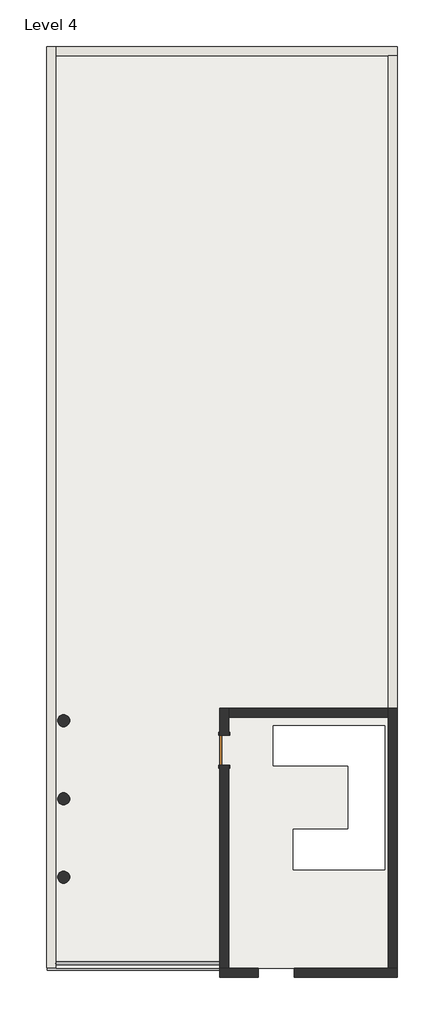
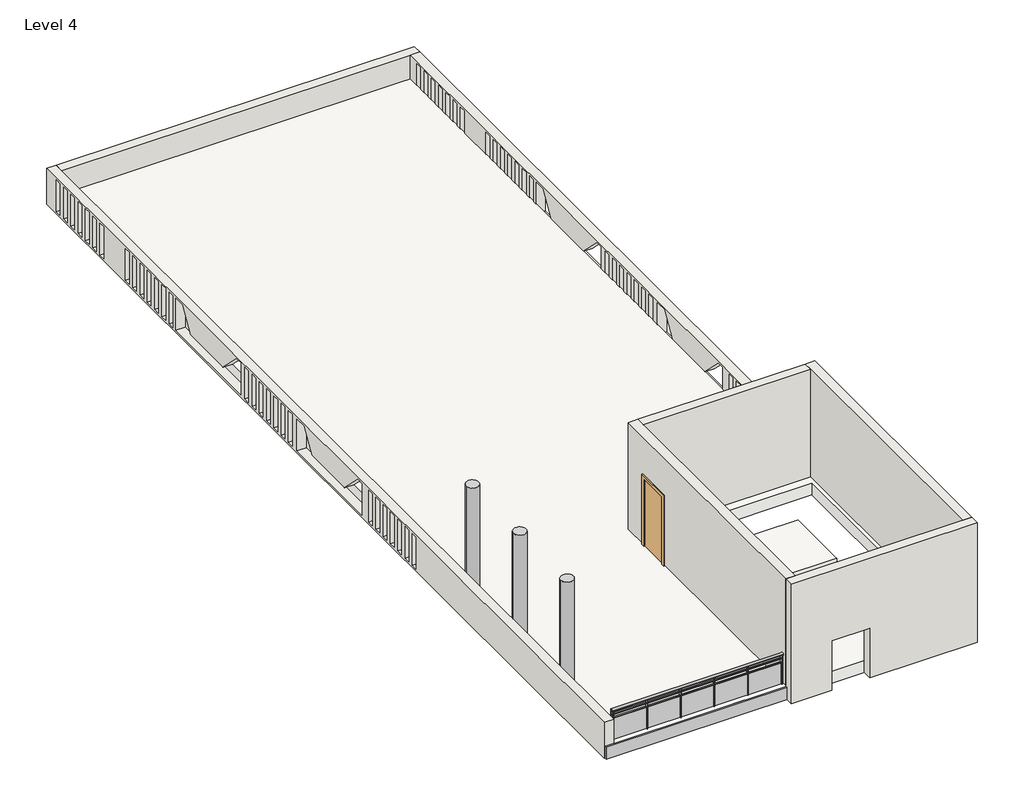
# One storey: 7 walls, 3 columns, 1 door, 1 proxy, 1 railing, 1 roof.
"""IFC4 building model written with IfcOpenShell, lengths in millimetres."""

from ifc_helpers import new_model, si_unit, point, frame, origin, place, context, project, spatial, polyline, ellipse_curve, trimmed, outline, extrude, faceted_brep, transform, mapped, element, save
from ifc_brep_helpers import plane_surface, extruded_surface, advanced_brep
from components import generic_models_12_generic_models_12_e4f72901, round_column_column_1_x_1_faae7945, door_a1484949

model = new_model("IFC4")

# Units and contexts
model_context = context("Model", 3, world=origin())
ifc_project = project(units=[si_unit("LENGTHUNIT", "METRE", prefix="MILLI")], contexts=[model_context])

# Site, building, storey
site = spatial("IfcSite", under=ifc_project)
building = spatial("IfcBuilding", under=site)
storey = spatial("IfcBuildingStorey", under=building, Name="Level 4", Elevation=6400.8)

# Proxy
placement = place(None, origin())
generic_models_12_generic_models_12_shape = generic_models_12_generic_models_12_e4f72901(model_context)
element("IfcBuildingElementProxy", 1, Name="Generic Models 12 : Generic Models 12", ObjectType="Generic Models 12 : Generic Models 12", at=placement, inside=storey, context=model_context, shape_type="MappedRepresentation", body=[
    mapped(generic_models_12_generic_models_12_shape, transform((0.0, 0.0, 0.0), x_axis=(1.0, 0.0, 0.0), y_axis=(0.0, 1.0, 0.0), z_axis=(0.0, 0.0, 1.0))),
])

# Columns
round_column_column_1_x_1_shape = round_column_column_1_x_1_faae7945(model_context)
element("IfcColumn", 2, ObjectType="Round Column : COLUMN 1' X 1'", at=placement, inside=storey, context=model_context, shape_type="MappedRepresentation", body=[
    mapped(round_column_column_1_x_1_shape, transform((1692.4423568, -10961.9073314, 0.0), x_axis=(1.0, 0.0, 0.0), y_axis=(0.0, 1.0, 0.0), z_axis=(0.0, 0.0, 1.0))),
])
element("IfcColumn", 3, ObjectType="Round Column : COLUMN 1' X 1'", at=placement, inside=storey, context=model_context, shape_type="MappedRepresentation", body=[
    mapped(round_column_column_1_x_1_shape, transform((1692.4423568, -6999.5073314, 0.0), x_axis=(1.0, 0.0, 0.0), y_axis=(0.0, 1.0, 0.0), z_axis=(0.0, 0.0, 1.0))),
])
element("IfcColumn", 4, ObjectType="Round Column : COLUMN 1' X 1'", at=placement, inside=storey, context=model_context, shape_type="MappedRepresentation", body=[
    mapped(round_column_column_1_x_1_shape, transform((1692.4423568, -8980.7073314, 0.0), x_axis=(1.0, 0.0, 0.0), y_axis=(0.0, 1.0, 0.0), z_axis=(0.0, 0.0, 1.0))),
])

# Door
door_shape = door_a1484949(model_context)
element("IfcDoor", 5, ObjectType="Single-Flush : 30\" x 80\"", at=placement, inside=storey, context=model_context, shape_type="MappedRepresentation", body=[
    mapped(door_shape, transform((5756.4423568, -7748.8073314, 6400.8), x_axis=(0.0, 1.0, 0.0), y_axis=(-1.0, 0.0, 0.0), z_axis=(0.0, 0.0, 1.0))),
])

# Railing
element("IfcRailing", 6, ObjectType="Glass Panel - Bottom Fill", at=placement, inside=storey, context=model_context, shape_type="SolidModel", body=[
    advanced_brep(
    [(1501.9423568, -13108.2073314, 7467.6), (1501.9423568, -13184.4073314, 7467.6), (5642.1423568, -13108.2073314, 7467.6), (5642.1423568, -13184.4073314, 7467.6)],
    [
        (0, 1, ellipse_curve(frame((1501.9423568, -13146.3073314, 7467.6), z_axis=(-1.0, 0.0, 0.0), x_axis=(0.0, -1.0, 0.0)), 38.1, 28.575)),
        (1, 0, ellipse_curve(frame((1501.9423568, -13146.3073314, 7467.6), z_axis=(-1.0, 0.0, 0.0), x_axis=(0.0, -1.0, 0.0)), 38.1, 28.575)),
        (2, 3, ellipse_curve(frame((5642.1423568, -13146.3073314, 7467.6), z_axis=(1.0, 0.0, 0.0), x_axis=(0.0, -1.0, 0.0)), 38.1, 28.575)),
        (3, 2, ellipse_curve(frame((5642.1423568, -13146.3073314, 7467.6), z_axis=(1.0, 0.0, 0.0), x_axis=(0.0, -1.0, 0.0)), 38.1, 28.575)),
        (0, 2),
        (3, 1),
    ],
    [
        plane_surface(frame((1501.9423568, -13146.3073314, 7467.6), z_axis=(-1.0, 0.0, 0.0), x_axis=(0.0, 1.0, 0.0))),
        plane_surface(frame((5642.1423568, -13146.3073314, 7467.6), z_axis=(1.0, 0.0, 0.0), x_axis=(0.0, 1.0, 0.0))),
        extruded_surface(trimmed(ellipse_curve(frame((5642.1423568, -13146.3073314, 7467.6), z_axis=(-1.0, 0.0, 0.0), x_axis=(0.0, -1.0, 0.0)), 38.1, 28.575), [point((5642.1423568, -13108.2073314, 7467.6))], [point((5642.1423568, -13184.4073314, 7467.6))], True, "CARTESIAN"), (-4140.2, 0.0, 0.0), 4140.2),
        extruded_surface(trimmed(ellipse_curve(frame((5642.1423568, -13146.3073314, 7467.6), z_axis=(-1.0, 0.0, 0.0), x_axis=(0.0, -1.0, 0.0)), 38.1, 28.575), [point((5642.1423568, -13184.4073314, 7467.6))], [point((5642.1423568, -13108.2073314, 7467.6))], True, "CARTESIAN"), (-4140.2, 0.0, 0.0), 4140.2),
    ],
    [
        (0, [[1, 2]]),
        (1, [[3, 4]]),
        (2, [[-1, 5, -4, 6]]),
        (3, [[-2, -6, -3, -5]]),
    ],
),
    extrude(outline(polyline([(1501.9423568, -13159.0073314), (1501.9423568, -13133.6073314), (5642.1423568, -13133.6073314), (5642.1423568, -13159.0073314), (1501.9423568, -13159.0073314)])), frame((0.0, 0.0, 7353.3), z_axis=(0.0, 0.0, 1.0), x_axis=(1.0, 0.0, 0.0)), (0.0, 0.0, 1.0), 25.4),
    extrude(outline(polyline([(1501.9423568, -13159.0073314), (1501.9423568, -13133.6073314), (5642.1423568, -13133.6073314), (5642.1423568, -13159.0073314), (1501.9423568, -13159.0073314)])), frame((0.0, 0.0, 7251.7), z_axis=(0.0, 0.0, 1.0), x_axis=(1.0, 0.0, 0.0)), (0.0, 0.0, 1.0), 25.4),
    extrude(outline(polyline([(5597.6923568, -13171.7073314), (5597.6923568, -13120.9073314), (5610.3923568, -13120.9073314), (5610.3923568, -13171.7073314), (5597.6923568, -13171.7073314)])), frame((0.0, 0.0, 6553.2), z_axis=(0.0, 0.0, 1.0), x_axis=(1.0, 0.0, 0.0)), (0.0, 0.0, 1.0), 885.825),
    extrude(outline(polyline([(4791.2423568, -13139.7721744), (5604.0423568, -13139.7721744), (5604.0423568, -13146.1221744), (4791.2423568, -13146.1221744), (4791.2423568, -13139.7721744)])), frame((0.0, 0.0, 6654.8), z_axis=(0.0, 0.0, 1.0), x_axis=(1.0, 0.0, 0.0)), (0.0, 0.0, 1.0), 596.9),
    extrude(outline(polyline([(4784.8923568, -13171.7073314), (4784.8923568, -13120.9073314), (4797.5923568, -13120.9073314), (4797.5923568, -13171.7073314), (4784.8923568, -13171.7073314)])), frame((0.0, 0.0, 6553.2), z_axis=(0.0, 0.0, 1.0), x_axis=(1.0, 0.0, 0.0)), (0.0, 0.0, 1.0), 885.825),
    extrude(outline(polyline([(3978.4423568, -13139.7721744), (4791.2423568, -13139.7721744), (4791.2423568, -13146.1221744), (3978.4423568, -13146.1221744), (3978.4423568, -13139.7721744)])), frame((0.0, 0.0, 6654.8), z_axis=(0.0, 0.0, 1.0), x_axis=(1.0, 0.0, 0.0)), (0.0, 0.0, 1.0), 596.9),
    extrude(outline(polyline([(3972.0923568, -13171.7073314), (3972.0923568, -13120.9073314), (3984.7923568, -13120.9073314), (3984.7923568, -13171.7073314), (3972.0923568, -13171.7073314)])), frame((0.0, 0.0, 6553.2), z_axis=(0.0, 0.0, 1.0), x_axis=(1.0, 0.0, 0.0)), (0.0, 0.0, 1.0), 885.825),
    extrude(outline(polyline([(3165.6423568, -13139.7721744), (3978.4423568, -13139.7721744), (3978.4423568, -13146.1221744), (3165.6423568, -13146.1221744), (3165.6423568, -13139.7721744)])), frame((0.0, 0.0, 6654.8), z_axis=(0.0, 0.0, 1.0), x_axis=(1.0, 0.0, 0.0)), (0.0, 0.0, 1.0), 596.9),
    extrude(outline(polyline([(3159.2923568, -13171.7073314), (3159.2923568, -13120.9073314), (3171.9923568, -13120.9073314), (3171.9923568, -13171.7073314), (3159.2923568, -13171.7073314)])), frame((0.0, 0.0, 6553.2), z_axis=(0.0, 0.0, 1.0), x_axis=(1.0, 0.0, 0.0)), (0.0, 0.0, 1.0), 885.825),
    extrude(outline(polyline([(2352.8423568, -13139.7721744), (3165.6423568, -13139.7721744), (3165.6423568, -13146.1221744), (2352.8423568, -13146.1221744), (2352.8423568, -13139.7721744)])), frame((0.0, 0.0, 6654.8), z_axis=(0.0, 0.0, 1.0), x_axis=(1.0, 0.0, 0.0)), (0.0, 0.0, 1.0), 596.9),
    extrude(outline(polyline([(2346.4923568, -13171.7073314), (2346.4923568, -13120.9073314), (2359.1923568, -13120.9073314), (2359.1923568, -13171.7073314), (2346.4923568, -13171.7073314)])), frame((0.0, 0.0, 6553.2), z_axis=(0.0, 0.0, 1.0), x_axis=(1.0, 0.0, 0.0)), (0.0, 0.0, 1.0), 885.825),
    extrude(outline(polyline([(1540.0423568, -13139.7721744), (2352.8423568, -13139.7721744), (2352.8423568, -13146.1221744), (1540.0423568, -13146.1221744), (1540.0423568, -13139.7721744)])), frame((0.0, 0.0, 6654.8), z_axis=(0.0, 0.0, 1.0), x_axis=(1.0, 0.0, 0.0)), (0.0, 0.0, 1.0), 596.9),
    extrude(outline(polyline([(1533.6923568, -13171.7073314), (1533.6923568, -13120.9073314), (1546.3923568, -13120.9073314), (1546.3923568, -13171.7073314), (1533.6923568, -13171.7073314)])), frame((0.0, 0.0, 6553.2), z_axis=(0.0, 0.0, 1.0), x_axis=(1.0, 0.0, 0.0)), (0.0, 0.0, 1.0), 885.825),
    extrude(outline(polyline([(5629.4423568, -13155.8323314), (5629.4423568, -13136.7823314), (5648.4923568, -13136.7823314), (5648.4923568, -13155.8323314), (5629.4423568, -13155.8323314)])), frame((0.0, 0.0, 6553.2), z_axis=(0.0, 0.0, 1.0), x_axis=(1.0, 0.0, 0.0)), (0.0, 0.0, 1.0), 885.825),
    extrude(outline(polyline([(1495.5923568, -13155.8323314), (1495.5923568, -13136.7823314), (1514.6423568, -13136.7823314), (1514.6423568, -13155.8323314), (1495.5923568, -13155.8323314)])), frame((0.0, 0.0, 6553.2), z_axis=(0.0, 0.0, 1.0), x_axis=(1.0, 0.0, 0.0)), (0.0, 0.0, 1.0), 885.825),
])

# Roof
element("IfcRoof", 7, ObjectType="ROOFING 6\"", at=placement, inside=storey, context=model_context, shape_type="SweptSolid", body=[
    extrude(outline(polyline([(1501.9423568, 9840.6926686), (9909.3423568, 9840.6926686), (9909.3423568, -13273.3073314), (1501.9423568, -13273.3073314), (1501.9423568, 9840.6926686)]), holes=[polyline([(7509.0423568, -9755.4073314), (7509.0423568, -10771.4073314), (9819.6463344, -10771.4073314), (9819.6463344, -7124.7746824), (7000.2463344, -7124.7746824), (7000.2463344, -8140.7746824), (8906.0423568, -8140.7746824), (8906.0423568, -9755.4073314), (7509.0423568, -9755.4073314)])]), frame((0.0, 0.0, 6400.8), z_axis=(0.0, 0.0, 1.0), x_axis=(1.0, 0.0, 0.0)), (0.0, 0.0, 1.0), 304.8),
])

# Walls
element("IfcWall", 8, ObjectType="OUTER WALL 9\"", at=placement, inside=storey, context=model_context, shape_type="Brep", body=[
    faceted_brep([(1489.2423568, 9840.6926686, 6400.8), (9909.3423568, 9840.6926686, 6400.8), (10137.9423568, 9840.6926686, 6400.8), (10137.9423568, 9840.6926686, 7315.2), (9909.3423568, 9840.6926686, 7315.2), (1489.2423568, 9840.6926686, 7315.2), (1489.2423568, 10069.2926686, 6400.8), (1489.2423568, 10069.2926686, 7315.2), (10137.9423568, 10069.2926686, 7315.2), (10137.9423568, 10069.2926686, 6400.8)], [[[0, 1, 2, 3, 4, 5]], [[6, 7, 8, 9]], [[2, 1, 0, 6, 9]], [[5, 4, 3, 8, 7]], [[3, 2, 9, 8]], [[0, 5, 7, 6]]]),
])
element("IfcWall", 9, ObjectType="OUTER WALL 9\"", at=placement, inside=storey, context=model_context, shape_type="Brep", body=[
    faceted_brep([(10137.9423568, -13501.9073314, 9448.8), (5642.1423568, -13501.9073314, 9448.8), (5642.1423568, -13501.9073314, 6400.8), (6619.47371, -13501.9073314, 6400.8), (6619.47371, -13501.9073314, 7669.779075), (7533.87371, -13501.9073314, 7669.779075), (7533.87371, -13501.9073314, 6400.8), (10137.9423568, -13501.9073314, 6400.8), (5642.1423568, -13273.3073314, 9448.8), (5870.7423568, -13273.3073314, 9448.8), (9909.3423568, -13273.3073314, 9448.8), (10137.9423568, -13273.3073314, 9448.8), (10137.9423568, -13273.3073314, 6400.8), (9909.3423568, -13273.3073314, 6400.8), (7533.87371, -13273.3073314, 6400.8), (7533.87371, -13273.3073314, 7669.779075), (6619.47371, -13273.3073314, 7669.779075), (6619.47371, -13273.3073314, 6400.8), (5642.1423568, -13273.3073314, 6400.8), (5642.1423568, -13273.3073314, 6729.4588212)], [[[0, 1, 2, 3, 4, 5, 6, 7]], [[8, 9, 10, 11, 12, 13, 14, 15, 16, 17, 18, 19]], [[12, 7, 6, 14, 13]], [[2, 18, 17, 3]], [[1, 0, 11, 10, 9, 8]], [[0, 7, 12, 11]], [[2, 1, 8, 19, 18]], [[16, 4, 3, 17]], [[4, 16, 15, 5]], [[5, 15, 14, 6]]]),
])
element("IfcWall", 10, ObjectType="OUTER WALL 9\"", at=placement, inside=storey, context=model_context, shape_type="Brep", body=[
    faceted_brep([(10137.9423568, -13273.3073314, 6400.8), (10137.9423568, -6689.1376827, 6400.8), (10137.9423568, -6689.1376827, 7315.2), (10137.9423568, -6689.1376827, 9448.8), (10137.9423568, -13273.3073314, 9448.8), (9909.3423568, -13273.3073314, 6400.8), (9909.3423568, -13273.3073314, 9448.8), (9909.3423568, -6917.7376827, 9448.8), (9909.3423568, -6689.1376827, 9448.8), (9909.3423568, -6689.1376827, 7315.2), (9909.3423568, -6689.1376827, 6400.8), (9909.3423568, -6917.7376827, 6400.8)], [[[0, 1, 2, 3, 4]], [[5, 6, 7, 8, 9, 10, 11]], [[1, 0, 5, 11, 10]], [[4, 3, 8, 7, 6]], [[0, 4, 6, 5]], [[1, 10, 9, 8, 3, 2]]]),
])
element("IfcWall", 11, ObjectType="OUTER WALL 9\"", at=placement, inside=storey, context=model_context, shape_type="Brep", body=[
    faceted_brep([(5642.1423568, -13273.3073314, 9448.8), (5642.1423568, -6689.1376827, 9448.8), (5642.1423568, -6689.1376827, 6729.4588212), (5642.1423568, -7367.8073314, 6729.4588212), (5642.1423568, -7367.8073314, 8432.8), (5642.1423568, -8129.8073314, 8432.8), (5642.1423568, -8129.8073314, 6729.4588212), (5642.1423568, -13273.3073314, 6729.4588212), (5870.7423568, -6689.1376827, 9448.8), (5870.7423568, -6917.7376827, 9448.8), (5870.7423568, -13273.3073314, 9448.8), (5870.7423568, -13273.3073314, 6729.4588212), (5870.7423568, -8129.8073314, 6729.4588212), (5870.7423568, -8129.8073314, 8432.8), (5870.7423568, -7367.8073314, 8432.8), (5870.7423568, -7367.8073314, 6729.4588212), (5870.7423568, -6689.1376827, 6729.4588212)], [[[0, 1, 2, 3, 4, 5, 6, 7]], [[8, 9, 10, 11, 12, 13, 14, 15, 16]], [[11, 7, 6, 12]], [[2, 16, 15, 3]], [[1, 0, 10, 9, 8]], [[0, 7, 11, 10]], [[14, 4, 3, 15]], [[4, 14, 13, 5]], [[5, 13, 12, 6]], [[2, 1, 8, 16]]]),
])
element("IfcWall", 12, ObjectType="OUTER WALL 9\"", at=placement, inside=storey, context=model_context, shape_type="Brep", body=[
    faceted_brep([(9909.3423568, -6689.1376827, 9448.8), (9909.3423568, -6689.1376827, 6400.8), (5870.7423568, -6689.1376827, 6400.8), (5870.7423568, -6689.1376827, 6729.4588212), (5870.7423568, -6689.1376827, 9448.8), (9909.3423568, -6917.7376827, 6400.8), (9909.3423568, -6917.7376827, 9448.8), (5870.7423568, -6917.7376827, 9448.8), (5870.7423568, -6917.7376827, 6400.8)], [[[0, 1, 2, 3, 4]], [[5, 6, 7, 8]], [[2, 1, 5, 8]], [[0, 4, 7, 6]], [[4, 3, 2, 8, 7]], [[0, 6, 5, 1]]]),
])
element("IfcWall", 13, ObjectType="OUTER WALL 9\"", at=placement, inside=storey, context=model_context, shape_type="SweptSolid", body=[
    extrude(outline(polyline([(9840.6926686, 6400.8), (-6689.1376827, 6400.8), (-6689.1376827, 7315.2), (9840.6926686, 7315.2), (9840.6926686, 6400.8)]), holes=[polyline([(-5335.8712555, 7264.4), (-5488.2712555, 7264.4), (-5488.2712555, 6451.6), (-5335.8712555, 6451.6), (-5335.8712555, 7264.4)]), polyline([(-5031.0712555, 7264.4), (-5183.4712555, 7264.4), (-5183.4712555, 6451.6), (-5031.0712555, 6451.6), (-5031.0712555, 7264.4)]), polyline([(-4726.2712555, 7264.4), (-4878.6712555, 7264.4), (-4878.6712555, 6451.6), (-4726.2712555, 6451.6), (-4726.2712555, 7264.4)]), polyline([(-4421.4712555, 7264.4), (-4573.8712555, 7264.4), (-4573.8712555, 6451.6), (-4421.4712555, 6451.6), (-4421.4712555, 7264.4)]), polyline([(-4116.6712555, 7264.4), (-4269.0712555, 7264.4), (-4269.0712555, 6451.6), (-4116.6712555, 6451.6), (-4116.6712555, 7264.4)]), polyline([(-3811.8712555, 7264.4), (-3964.2712555, 7264.4), (-3964.2712555, 6451.6), (-3811.8712555, 6451.6), (-3811.8712555, 7264.4)]), polyline([(-3507.0712555, 7264.4), (-3659.4712555, 7264.4), (-3659.4712555, 6451.6), (-3507.0712555, 6451.6), (-3507.0712555, 7264.4)]), polyline([(-154.2712555, 7264.4), (-306.6712555, 7264.4), (-306.6712555, 6451.6), (-154.2712555, 6451.6), (-154.2712555, 7264.4)]), polyline([(150.5287445, 7264.4), (-1.8712555, 7264.4), (-1.8712555, 6451.6), (150.5287445, 6451.6), (150.5287445, 7264.4)]), polyline([(455.3287445, 7264.4), (302.9287445, 7264.4), (302.9287445, 6451.6), (455.3287445, 6451.6), (455.3287445, 7264.4)]), polyline([(760.1287445, 7264.4), (607.7287445, 7264.4), (607.7287445, 6451.6), (760.1287445, 6451.6), (760.1287445, 7264.4)]), polyline([(1064.9287445, 7264.4), (912.5287445, 7264.4), (912.5287445, 6451.6), (1064.9287445, 6451.6), (1064.9287445, 7264.4)]), polyline([(1369.7287445, 7264.4), (1217.3287445, 7264.4), (1217.3287445, 6451.6), (1369.7287445, 6451.6), (1369.7287445, 7264.4)]), polyline([(1674.5287445, 7264.4), (1522.1287445, 7264.4), (1522.1287445, 6451.6), (1674.5287445, 6451.6), (1674.5287445, 7264.4)]), polyline([(4836.8926686, 7264.4), (4684.4926686, 7264.4), (4684.4926686, 6451.6), (4836.8926686, 6451.6), (4836.8926686, 7264.4)]), polyline([(5141.6926686, 7264.4), (4989.2926686, 7264.4), (4989.2926686, 6451.6), (5141.6926686, 6451.6), (5141.6926686, 7264.4)]), polyline([(5446.4926686, 7264.4), (5294.0926686, 7264.4), (5294.0926686, 6451.6), (5446.4926686, 6451.6), (5446.4926686, 7264.4)]), polyline([(5751.2926686, 7264.4), (5598.8926686, 7264.4), (5598.8926686, 6451.6), (5751.2926686, 6451.6), (5751.2926686, 7264.4)]), polyline([(6056.0926686, 7264.4), (5903.6926686, 7264.4), (5903.6926686, 6451.6), (6056.0926686, 6451.6), (6056.0926686, 7264.4)]), polyline([(6360.8926686, 7264.4), (6208.4926686, 7264.4), (6208.4926686, 6451.6), (6360.8926686, 6451.6), (6360.8926686, 7264.4)]), polyline([(6665.6926686, 7264.4), (6513.2926686, 7264.4), (6513.2926686, 6451.6), (6665.6926686, 6451.6), (6665.6926686, 7264.4)]), polyline([(7732.4926686, 7264.4), (7580.0926686, 7264.4), (7580.0926686, 6451.6), (7732.4926686, 6451.6), (7732.4926686, 7264.4)]), polyline([(8037.2926686, 7264.4), (7884.8926686, 7264.4), (7884.8926686, 6451.6), (8037.2926686, 6451.6), (8037.2926686, 7264.4)]), polyline([(8342.0926686, 7264.4), (8189.6926686, 7264.4), (8189.6926686, 6451.6), (8342.0926686, 6451.6), (8342.0926686, 7264.4)]), polyline([(8646.8926686, 7264.4), (8494.4926686, 7264.4), (8494.4926686, 6451.6), (8646.8926686, 6451.6), (8646.8926686, 7264.4)]), polyline([(8951.6926686, 7264.4), (8799.2926686, 7264.4), (8799.2926686, 6451.6), (8951.6926686, 6451.6), (8951.6926686, 7264.4)]), polyline([(9256.4926686, 7264.4), (9104.0926686, 7264.4), (9104.0926686, 6451.6), (9256.4926686, 6451.6), (9256.4926686, 7264.4)]), polyline([(9561.2926686, 7264.4), (9408.8926686, 7264.4), (9408.8926686, 6451.6), (9561.2926686, 6451.6), (9561.2926686, 7264.4)]), polyline([(-2491.0073314, 6705.6), (-3049.8073314, 7264.4), (-3227.6712555, 7264.4), (-3227.6712555, 6451.6), (-509.8712555, 6451.6), (-509.8712555, 7264.4), (-783.6464175, 7264.4), (-1119.4073314, 6705.6), (-2491.0073314, 6705.6)]), polyline([(2588.9926686, 6705.6), (2030.1926686, 7264.4), (1852.3287445, 7264.4), (1852.3287445, 6451.6), (4570.1287445, 6451.6), (4570.1287445, 7264.4), (4296.3535825, 7264.4), (3960.5926686, 6705.6), (2588.9926686, 6705.6)])]), frame((9909.3423568, 0.0, 0.0), z_axis=(1.0, 0.0, 0.0), x_axis=(0.0, 1.0, 0.0)), (0.0, 0.0, 1.0), 228.6),
])
element("IfcWall", 14, ObjectType="OUTER WALL 9\"", at=placement, inside=storey, context=model_context, shape_type="Brep", body=[
    faceted_brep([(1260.6423568, 10069.2926686, 6400.8), (1260.6423568, -13260.6073314, 6400.8), (1260.6423568, -13260.6073314, 7315.2), (1260.6423568, 10069.2926686, 7315.2), (1260.6423568, -5234.2712555, 7264.4), (1260.6423568, -5386.6712555, 7264.4), (1260.6423568, -5386.6712555, 6451.6), (1260.6423568, -5234.2712555, 6451.6), (1260.6423568, -4929.4712555, 7264.4), (1260.6423568, -5081.8712555, 7264.4), (1260.6423568, -5081.8712555, 6451.6), (1260.6423568, -4929.4712555, 6451.6), (1260.6423568, -4624.6712555, 7264.4), (1260.6423568, -4777.0712555, 7264.4), (1260.6423568, -4777.0712555, 6451.6), (1260.6423568, -4624.6712555, 6451.6), (1260.6423568, -4319.8712555, 7264.4), (1260.6423568, -4472.2712555, 7264.4), (1260.6423568, -4472.2712555, 6451.6), (1260.6423568, -4319.8712555, 6451.6), (1260.6423568, -4015.0712555, 7264.4), (1260.6423568, -4167.4712555, 7264.4), (1260.6423568, -4167.4712555, 6451.6), (1260.6423568, -4015.0712555, 6451.6), (1260.6423568, -3710.2712555, 7264.4), (1260.6423568, -3862.6712555, 7264.4), (1260.6423568, -3862.6712555, 6451.6), (1260.6423568, -3710.2712555, 6451.6), (1260.6423568, -3405.4712555, 7264.4), (1260.6423568, -3557.8712555, 7264.4), (1260.6423568, -3557.8712555, 6451.6), (1260.6423568, -3405.4712555, 6451.6), (1260.6423568, -52.6712555, 7264.4), (1260.6423568, -205.0712555, 7264.4), (1260.6423568, -205.0712555, 6451.6), (1260.6423568, -52.6712555, 6451.6), (1260.6423568, 252.1287445, 7264.4), (1260.6423568, 99.7287445, 7264.4), (1260.6423568, 99.7287445, 6451.6), (1260.6423568, 252.1287445, 6451.6), (1260.6423568, 556.9287445, 7264.4), (1260.6423568, 404.5287445, 7264.4), (1260.6423568, 404.5287445, 6451.6), (1260.6423568, 556.9287445, 6451.6), (1260.6423568, 861.7287445, 7264.4), (1260.6423568, 709.3287445, 7264.4), (1260.6423568, 709.3287445, 6451.6), (1260.6423568, 861.7287445, 6451.6), (1260.6423568, 1166.5287445, 7264.4), (1260.6423568, 1014.1287445, 7264.4), (1260.6423568, 1014.1287445, 6451.6), (1260.6423568, 1166.5287445, 6451.6), (1260.6423568, 1471.3287445, 7264.4), (1260.6423568, 1318.9287445, 7264.4), (1260.6423568, 1318.9287445, 6451.6), (1260.6423568, 1471.3287445, 6451.6), (1260.6423568, 1776.1287445, 7264.4), (1260.6423568, 1623.7287445, 7264.4), (1260.6423568, 1623.7287445, 6451.6), (1260.6423568, 1776.1287445, 6451.6), (1260.6423568, 4938.4926686, 7264.4), (1260.6423568, 4786.0926686, 7264.4), (1260.6423568, 4786.0926686, 6451.6), (1260.6423568, 4938.4926686, 6451.6), (1260.6423568, 5243.2926686, 7264.4), (1260.6423568, 5090.8926686, 7264.4), (1260.6423568, 5090.8926686, 6451.6), (1260.6423568, 5243.2926686, 6451.6), (1260.6423568, 5548.0926686, 7264.4), (1260.6423568, 5395.6926686, 7264.4), (1260.6423568, 5395.6926686, 6451.6), (1260.6423568, 5548.0926686, 6451.6), (1260.6423568, 5852.8926686, 7264.4), (1260.6423568, 5700.4926686, 7264.4), (1260.6423568, 5700.4926686, 6451.6), (1260.6423568, 5852.8926686, 6451.6), (1260.6423568, 6157.6926686, 7264.4), (1260.6423568, 6005.2926686, 7264.4), (1260.6423568, 6005.2926686, 6451.6), (1260.6423568, 6157.6926686, 6451.6), (1260.6423568, 6462.4926686, 7264.4), (1260.6423568, 6310.0926686, 7264.4), (1260.6423568, 6310.0926686, 6451.6), (1260.6423568, 6462.4926686, 6451.6), (1260.6423568, 6767.2926686, 7264.4), (1260.6423568, 6614.8926686, 7264.4), (1260.6423568, 6614.8926686, 6451.6), (1260.6423568, 6767.2926686, 6451.6), (1260.6423568, 7834.0926686, 7264.4), (1260.6423568, 7681.6926686, 7264.4), (1260.6423568, 7681.6926686, 6451.6), (1260.6423568, 7834.0926686, 6451.6), (1260.6423568, 8138.8926686, 7264.4), (1260.6423568, 7986.4926686, 7264.4), (1260.6423568, 7986.4926686, 6451.6), (1260.6423568, 8138.8926686, 6451.6), (1260.6423568, 8443.6926686, 7264.4), (1260.6423568, 8291.2926686, 7264.4), (1260.6423568, 8291.2926686, 6451.6), (1260.6423568, 8443.6926686, 6451.6), (1260.6423568, 8748.4926686, 7264.4), (1260.6423568, 8596.0926686, 7264.4), (1260.6423568, 8596.0926686, 6451.6), (1260.6423568, 8748.4926686, 6451.6), (1260.6423568, 9053.2926686, 7264.4), (1260.6423568, 8900.8926686, 7264.4), (1260.6423568, 8900.8926686, 6451.6), (1260.6423568, 9053.2926686, 6451.6), (1260.6423568, 9358.0926686, 7264.4), (1260.6423568, 9205.6926686, 7264.4), (1260.6423568, 9205.6926686, 6451.6), (1260.6423568, 9358.0926686, 6451.6), (1260.6423568, 9662.8926686, 7264.4), (1260.6423568, 9510.4926686, 7264.4), (1260.6423568, 9510.4926686, 6451.6), (1260.6423568, 9662.8926686, 6451.6), (1260.6423568, -2389.4073314, 6705.6), (1260.6423568, -2948.2073314, 7264.4), (1260.6423568, -3126.0712555, 7264.4), (1260.6423568, -3126.0712555, 6451.6), (1260.6423568, -408.2712555, 6451.6), (1260.6423568, -408.2712555, 7264.4), (1260.6423568, -682.0464175, 7264.4), (1260.6423568, -1017.8073314, 6705.6), (1260.6423568, 2690.5926686, 6705.6), (1260.6423568, 2131.7926686, 7264.4), (1260.6423568, 1953.9287445, 7264.4), (1260.6423568, 1953.9287445, 6451.6), (1260.6423568, 4671.7287445, 6451.6), (1260.6423568, 4671.7287445, 7264.4), (1260.6423568, 4397.9535825, 7264.4), (1260.6423568, 4062.1926686, 6705.6), (1489.2423568, 10069.2926686, 6400.8), (1489.2423568, 10069.2926686, 7315.2), (1489.2423568, 9840.6926686, 7315.2), (1489.2423568, -13260.6073314, 7315.2), (1489.2423568, -13260.6073314, 6400.8), (1489.2423568, 9840.6926686, 6400.8), (1489.2423568, -5234.2712555, 7264.4), (1489.2423568, -5234.2712555, 6451.6), (1489.2423568, -5386.6712555, 6451.6), (1489.2423568, -5386.6712555, 7264.4), (1489.2423568, -4929.4712555, 7264.4), (1489.2423568, -4929.4712555, 6451.6), (1489.2423568, -5081.8712555, 6451.6), (1489.2423568, -5081.8712555, 7264.4), (1489.2423568, -4624.6712555, 7264.4), (1489.2423568, -4624.6712555, 6451.6), (1489.2423568, -4777.0712555, 6451.6), (1489.2423568, -4777.0712555, 7264.4), (1489.2423568, -4319.8712555, 7264.4), (1489.2423568, -4319.8712555, 6451.6), (1489.2423568, -4472.2712555, 6451.6), (1489.2423568, -4472.2712555, 7264.4), (1489.2423568, -4015.0712555, 7264.4), (1489.2423568, -4015.0712555, 6451.6), (1489.2423568, -4167.4712555, 6451.6), (1489.2423568, -4167.4712555, 7264.4), (1489.2423568, -3710.2712555, 7264.4), (1489.2423568, -3710.2712555, 6451.6), (1489.2423568, -3862.6712555, 6451.6), (1489.2423568, -3862.6712555, 7264.4), (1489.2423568, -3405.4712555, 7264.4), (1489.2423568, -3405.4712555, 6451.6), (1489.2423568, -3557.8712555, 6451.6), (1489.2423568, -3557.8712555, 7264.4), (1489.2423568, -52.6712555, 7264.4), (1489.2423568, -52.6712555, 6451.6), (1489.2423568, -205.0712555, 6451.6), (1489.2423568, -205.0712555, 7264.4), (1489.2423568, 252.1287445, 7264.4), (1489.2423568, 252.1287445, 6451.6), (1489.2423568, 99.7287445, 6451.6), (1489.2423568, 99.7287445, 7264.4), (1489.2423568, 556.9287445, 7264.4), (1489.2423568, 556.9287445, 6451.6), (1489.2423568, 404.5287445, 6451.6), (1489.2423568, 404.5287445, 7264.4), (1489.2423568, 861.7287445, 7264.4), (1489.2423568, 861.7287445, 6451.6), (1489.2423568, 709.3287445, 6451.6), (1489.2423568, 709.3287445, 7264.4), (1489.2423568, 1166.5287445, 7264.4), (1489.2423568, 1166.5287445, 6451.6), (1489.2423568, 1014.1287445, 6451.6), (1489.2423568, 1014.1287445, 7264.4), (1489.2423568, 1471.3287445, 7264.4), (1489.2423568, 1471.3287445, 6451.6), (1489.2423568, 1318.9287445, 6451.6), (1489.2423568, 1318.9287445, 7264.4), (1489.2423568, 1776.1287445, 7264.4), (1489.2423568, 1776.1287445, 6451.6), (1489.2423568, 1623.7287445, 6451.6), (1489.2423568, 1623.7287445, 7264.4), (1489.2423568, 4938.4926686, 7264.4), (1489.2423568, 4938.4926686, 6451.6), (1489.2423568, 4786.0926686, 6451.6), (1489.2423568, 4786.0926686, 7264.4), (1489.2423568, 5243.2926686, 7264.4), (1489.2423568, 5243.2926686, 6451.6), (1489.2423568, 5090.8926686, 6451.6), (1489.2423568, 5090.8926686, 7264.4), (1489.2423568, 5548.0926686, 7264.4), (1489.2423568, 5548.0926686, 6451.6), (1489.2423568, 5395.6926686, 6451.6), (1489.2423568, 5395.6926686, 7264.4), (1489.2423568, 5852.8926686, 7264.4), (1489.2423568, 5852.8926686, 6451.6), (1489.2423568, 5700.4926686, 6451.6), (1489.2423568, 5700.4926686, 7264.4), (1489.2423568, 6157.6926686, 7264.4), (1489.2423568, 6157.6926686, 6451.6), (1489.2423568, 6005.2926686, 6451.6), (1489.2423568, 6005.2926686, 7264.4), (1489.2423568, 6462.4926686, 7264.4), (1489.2423568, 6462.4926686, 6451.6), (1489.2423568, 6310.0926686, 6451.6), (1489.2423568, 6310.0926686, 7264.4), (1489.2423568, 6767.2926686, 7264.4), (1489.2423568, 6767.2926686, 6451.6), (1489.2423568, 6614.8926686, 6451.6), (1489.2423568, 6614.8926686, 7264.4), (1489.2423568, 7834.0926686, 7264.4), (1489.2423568, 7834.0926686, 6451.6), (1489.2423568, 7681.6926686, 6451.6), (1489.2423568, 7681.6926686, 7264.4), (1489.2423568, 8138.8926686, 7264.4), (1489.2423568, 8138.8926686, 6451.6), (1489.2423568, 7986.4926686, 6451.6), (1489.2423568, 7986.4926686, 7264.4), (1489.2423568, 8443.6926686, 7264.4), (1489.2423568, 8443.6926686, 6451.6), (1489.2423568, 8291.2926686, 6451.6), (1489.2423568, 8291.2926686, 7264.4), (1489.2423568, 8748.4926686, 7264.4), (1489.2423568, 8748.4926686, 6451.6), (1489.2423568, 8596.0926686, 6451.6), (1489.2423568, 8596.0926686, 7264.4), (1489.2423568, 9053.2926686, 7264.4), (1489.2423568, 9053.2926686, 6451.6), (1489.2423568, 8900.8926686, 6451.6), (1489.2423568, 8900.8926686, 7264.4), (1489.2423568, 9358.0926686, 7264.4), (1489.2423568, 9358.0926686, 6451.6), (1489.2423568, 9205.6926686, 6451.6), (1489.2423568, 9205.6926686, 7264.4), (1489.2423568, 9662.8926686, 7264.4), (1489.2423568, 9662.8926686, 6451.6), (1489.2423568, 9510.4926686, 6451.6), (1489.2423568, 9510.4926686, 7264.4), (1489.2423568, -2389.4073314, 6705.6), (1489.2423568, -1017.8073314, 6705.6), (1489.2423568, -682.0464175, 7264.4), (1489.2423568, -408.2712555, 7264.4), (1489.2423568, -408.2712555, 6451.6), (1489.2423568, -3126.0712555, 6451.6), (1489.2423568, -3126.0712555, 7264.4), (1489.2423568, -2948.2073314, 7264.4), (1489.2423568, 2690.5926686, 6705.6), (1489.2423568, 4062.1926686, 6705.6), (1489.2423568, 4397.9535825, 7264.4), (1489.2423568, 4671.7287445, 7264.4), (1489.2423568, 4671.7287445, 6451.6), (1489.2423568, 1953.9287445, 6451.6), (1489.2423568, 1953.9287445, 7264.4), (1489.2423568, 2131.7926686, 7264.4)], [[[0, 1, 2, 3], [4, 5, 6, 7], [8, 9, 10, 11], [12, 13, 14, 15], [16, 17, 18, 19], [20, 21, 22, 23], [24, 25, 26, 27], [28, 29, 30, 31], [32, 33, 34, 35], [36, 37, 38, 39], [40, 41, 42, 43], [44, 45, 46, 47], [48, 49, 50, 51], [52, 53, 54, 55], [56, 57, 58, 59], [60, 61, 62, 63], [64, 65, 66, 67], [68, 69, 70, 71], [72, 73, 74, 75], [76, 77, 78, 79], [80, 81, 82, 83], [84, 85, 86, 87], [88, 89, 90, 91], [92, 93, 94, 95], [96, 97, 98, 99], [100, 101, 102, 103], [104, 105, 106, 107], [108, 109, 110, 111], [112, 113, 114, 115], [116, 117, 118, 119, 120, 121, 122, 123], [124, 125, 126, 127, 128, 129, 130, 131]], [[132, 133, 134, 135, 136, 137], [138, 139, 140, 141], [142, 143, 144, 145], [146, 147, 148, 149], [150, 151, 152, 153], [154, 155, 156, 157], [158, 159, 160, 161], [162, 163, 164, 165], [166, 167, 168, 169], [170, 171, 172, 173], [174, 175, 176, 177], [178, 179, 180, 181], [182, 183, 184, 185], [186, 187, 188, 189], [190, 191, 192, 193], [194, 195, 196, 197], [198, 199, 200, 201], [202, 203, 204, 205], [206, 207, 208, 209], [210, 211, 212, 213], [214, 215, 216, 217], [218, 219, 220, 221], [222, 223, 224, 225], [226, 227, 228, 229], [230, 231, 232, 233], [234, 235, 236, 237], [238, 239, 240, 241], [242, 243, 244, 245], [246, 247, 248, 249], [250, 251, 252, 253, 254, 255, 256, 257], [258, 259, 260, 261, 262, 263, 264, 265]], [[1, 0, 132, 137, 136]], [[2, 1, 136, 135]], [[3, 2, 135, 134, 133]], [[5, 4, 138, 141]], [[6, 5, 141, 140]], [[7, 6, 140, 139]], [[4, 7, 139, 138]], [[9, 8, 142, 145]], [[10, 9, 145, 144]], [[11, 10, 144, 143]], [[8, 11, 143, 142]], [[13, 12, 146, 149]], [[14, 13, 149, 148]], [[15, 14, 148, 147]], [[12, 15, 147, 146]], [[17, 16, 150, 153]], [[18, 17, 153, 152]], [[19, 18, 152, 151]], [[16, 19, 151, 150]], [[21, 20, 154, 157]], [[22, 21, 157, 156]], [[23, 22, 156, 155]], [[20, 23, 155, 154]], [[25, 24, 158, 161]], [[26, 25, 161, 160]], [[27, 26, 160, 159]], [[24, 27, 159, 158]], [[29, 28, 162, 165]], [[30, 29, 165, 164]], [[31, 30, 164, 163]], [[28, 31, 163, 162]], [[33, 32, 166, 169]], [[34, 33, 169, 168]], [[35, 34, 168, 167]], [[32, 35, 167, 166]], [[37, 36, 170, 173]], [[38, 37, 173, 172]], [[39, 38, 172, 171]], [[36, 39, 171, 170]], [[41, 40, 174, 177]], [[42, 41, 177, 176]], [[43, 42, 176, 175]], [[40, 43, 175, 174]], [[45, 44, 178, 181]], [[46, 45, 181, 180]], [[47, 46, 180, 179]], [[44, 47, 179, 178]], [[49, 48, 182, 185]], [[50, 49, 185, 184]], [[51, 50, 184, 183]], [[48, 51, 183, 182]], [[53, 52, 186, 189]], [[54, 53, 189, 188]], [[55, 54, 188, 187]], [[52, 55, 187, 186]], [[57, 56, 190, 193]], [[58, 57, 193, 192]], [[59, 58, 192, 191]], [[56, 59, 191, 190]], [[61, 60, 194, 197]], [[62, 61, 197, 196]], [[63, 62, 196, 195]], [[60, 63, 195, 194]], [[65, 64, 198, 201]], [[66, 65, 201, 200]], [[67, 66, 200, 199]], [[64, 67, 199, 198]], [[69, 68, 202, 205]], [[70, 69, 205, 204]], [[71, 70, 204, 203]], [[68, 71, 203, 202]], [[73, 72, 206, 209]], [[74, 73, 209, 208]], [[75, 74, 208, 207]], [[72, 75, 207, 206]], [[77, 76, 210, 213]], [[78, 77, 213, 212]], [[79, 78, 212, 211]], [[76, 79, 211, 210]], [[81, 80, 214, 217]], [[82, 81, 217, 216]], [[83, 82, 216, 215]], [[80, 83, 215, 214]], [[85, 84, 218, 221]], [[86, 85, 221, 220]], [[87, 86, 220, 219]], [[84, 87, 219, 218]], [[89, 88, 222, 225]], [[90, 89, 225, 224]], [[91, 90, 224, 223]], [[88, 91, 223, 222]], [[93, 92, 226, 229]], [[94, 93, 229, 228]], [[95, 94, 228, 227]], [[92, 95, 227, 226]], [[97, 96, 230, 233]], [[98, 97, 233, 232]], [[99, 98, 232, 231]], [[96, 99, 231, 230]], [[101, 100, 234, 237]], [[102, 101, 237, 236]], [[103, 102, 236, 235]], [[100, 103, 235, 234]], [[105, 104, 238, 241]], [[106, 105, 241, 240]], [[107, 106, 240, 239]], [[104, 107, 239, 238]], [[109, 108, 242, 245]], [[110, 109, 245, 244]], [[111, 110, 244, 243]], [[108, 111, 243, 242]], [[113, 112, 246, 249]], [[114, 113, 249, 248]], [[115, 114, 248, 247]], [[112, 115, 247, 246]], [[117, 116, 250, 257]], [[118, 117, 257, 256]], [[119, 118, 256, 255]], [[120, 119, 255, 254]], [[121, 120, 254, 253]], [[122, 121, 253, 252]], [[123, 122, 252, 251]], [[116, 123, 251, 250]], [[125, 124, 258, 265]], [[126, 125, 265, 264]], [[127, 126, 264, 263]], [[128, 127, 263, 262]], [[129, 128, 262, 261]], [[130, 129, 261, 260]], [[131, 130, 260, 259]], [[124, 131, 259, 258]], [[0, 3, 133, 132]]]),
])

save(model, "model.ifc")

# Revit data of these elements
# Type "Round Column : COLUMN 1' X 1'"
#   Assembly Code = "B1010200"
#   Diameter = 1' - 0"
#   Offset Base = 0' - 0"
#   Offset Top = 0' - 0"
#   Material = CREAM BEIGE COLOUR
# Type "Single-Flush : 30\" x 80\""
#   Type Mark = "5"
#   Construction Type Id = "MDOOR"
#   Assembly Code = "C1020"
#   Analytic Construction = "Metal"
#   Thickness = 0' - 2"
#   Heat Transfer Coefficient (U) = 0.651978 BTU/(h·ft²·°F)
#   Height = 6' - 8"
#   Trim Projection Ext = 0' - 1"
#   Trim Projection Int = 0' - 1"
#   Trim Width = 0' - 3"
#   Width = 2' - 6"
#   Define Thermal Properties by = 1
#   Define Thermal Properties by = 1
#   Door Material = Door - Panel
#   Frame Material = Door - Frame
#   Visual Light Transmittance = 0
#   Solar Heat Gain Coefficient = 0
#   Function = (empty or 0)
#   Wall Closure = (empty or 0)
# Type "Glass Panel - Bottom Fill"
#   Assembly Code = "C2010400"
#   built-in parameter 1008612 = 0.0416667 (stored number, unit not read)
#   built-in parameter 1008611 = 0.0416667 (stored number, unit not read)
#   built-in parameter 1008609 = 0.333333 (stored number, unit not read)
#   built-in parameter 1008604 = 0.166667 (stored number, unit not read)
#   built-in parameter 1008603 = 0.166667 (stored number, unit not read)
#   Railing Height = 3' - 0"
#   built-in parameter 1008630 = 2
#   built-in parameter 1008610 = 2
#   built-in parameter 1008618 = Baluster - Square : 3/4"
# Type "ROOFING 6\""
#   Assembly Code = "B1020"
#   Layers, outside or top first: 1' - 0" "ROOFING 6\"" (function 1)
# Type "OUTER WALL 9\""
#   Assembly Code = "B2010"
#   Layers, outside or top first: 0' - 9" "CREAM BEIGE COLOUR" (function 1)
# Element 1 (IfcBuildingElementProxy, "Generic Models 12 : Generic Models 12")
#   Phase Created = New Construction
#   Materials on its faces: "Clad - White"
# Elements 2, 3, 4 (IfcColumn, "Round Column : COLUMN 1' X 1'")
#   Phase Created = New Construction
#   Materials on its faces: "CREAM BEIGE COLOUR"
# Element 5 (IfcDoor, "Single-Flush : 30\" x 80\"")
#   Phase Created = New Construction
#   Materials on its faces: "Door - Frame", "Door - Panel"
# Element 6 (IfcRailing, "Glass Panel - Bottom Fill")
#   built-in parameter 1008621 = 0.5 (stored number, unit not read)
#   Phase Created = New Construction
#   Materials on its faces: "Glass"
# Element 7 (IfcRoof, "ROOFING 6\"")
#   built-in parameter 1001705 = 22 (stored number, unit not read)
#   built-in parameter 1001710 = 33615
#   Phase Created = New Construction
#   Materials on its faces: "ROOFING 6\""
# Elements 8, 13, 14 (IfcWall, "OUTER WALL 9\"")
#   Top Offset = 0' - 0"
#   Base Offset = 0' - 0"
#   Unconnected Height = 3' - 0"
#   wall height = 3' - 0"
#   Phase Created = New Construction
#   Base Constraint = Level 4
#   Materials on its faces: "CREAM BEIGE COLOUR"
# Elements 9, 10 (IfcWall, "OUTER WALL 9\"")
#   Top Offset = 0' - 0"
#   Base Offset = 0' - 0"
#   Unconnected Height = 10' - 0"
#   wall height = 10' - 0"
#   Phase Created = New Construction
#   Base Constraint = Level 4
#   Materials on its faces: "CREAM BEIGE COLOUR"
# Element 11 (IfcWall, "OUTER WALL 9\"")
#   built-in parameter 1001111 = 1' - 0.93932"
#   Top Offset = 0' - 0"
#   Base Offset = 1' - 0.93932"
#   Unconnected Height = 8' - 11.06068"
#   wall height = 8' - 11.06068"
#   Phase Created = New Construction
#   Base Constraint = Level 4
#   Materials on its faces: "CREAM BEIGE COLOUR"
# Element 12 (IfcWall, "OUTER WALL 9\"")
#   Top Offset = 0' - 0"
#   Base Offset = 0' - 0"
#   wall height = 10' - 0"
#   Phase Created = New Construction
#   Base Constraint = Level 4
#   Top Constraint = HEAD ROOM
#   Materials on its faces: "CREAM BEIGE COLOUR"
# Materials
#   "CREAM BEIGE COLOUR": class "Generic", colour RGB 120 120 120, transparency 0, Cost = 0
#   "Door - Panel": class "Wood", colour RGB 210 159 95, transparency 0, Cost = 0
#   "Door - Frame": colour RGB 118 70 51, transparency 0, Cost = 0
#   "ROOFING 6\"": class "Generic", colour RGB 120 120 120, transparency 0, Cost = 0
#   "Clad - White": class "Wood", colour RGB 242 242 238, transparency 0, Cost = 0
#   "Glass": class "Glass", colour RGB 0 128 192, transparency 0.75, Description = "Soda Lime Glass", Cost = 0
